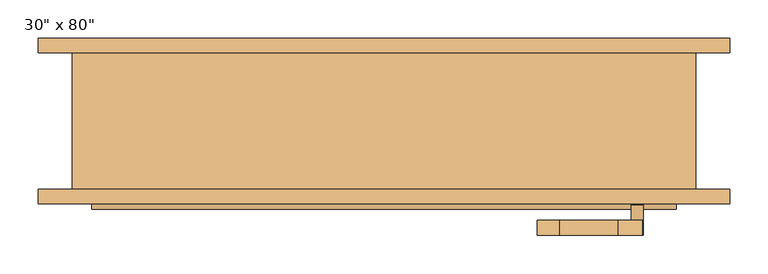
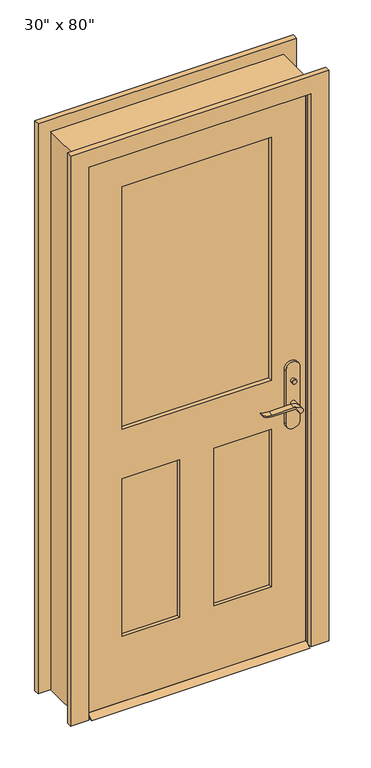
"""IFC4 building model written with IfcOpenShell, lengths in millimetres: door geometry."""

from ifc_helpers import new_model, si_unit, point, frame, frame_2d, origin, place, context, project, spatial, polyline, circle_curve, trimmed, segment, composite_curve, outline, extrude, faceted_brep, source, transform, mapped, element, save


def door_3dfc5bb7(model_context):
    return source(origin(), model_context, "Body", "SolidModel", [
        extrude(outline(polyline([(-50.8, 12.7), (-25.4, 0.0), (-111.125, 0.0), (-85.725, 12.7), (-50.8, 12.7)])), frame((-381.0, 0.0, 0.0), z_axis=(1.0, 0.0, 0.0), x_axis=(0.0, 1.0, 0.0)), (0.0, 0.0, 1.0), 762.0),
        extrude(outline(polyline([(335.2, -30.8), (335.2, -40.8), (325.2, -40.8), (325.2, -30.8), (335.2, -30.8)])), frame((0.0, 0.0, 981.9), z_axis=(0.0, 0.0, 1.0), x_axis=(1.0, 0.0, 0.0)), (0.0, 0.0, 1.0), 30.0),
        extrude(outline(composite_curve([segment(trimmed(circle_curve(frame_2d((996.9, 330.2)), 8.0), [point((996.9, 322.2))], [point((996.9, 338.2))], False, "CARTESIAN"), True, "CONTINUOUS"), segment(trimmed(circle_curve(frame_2d((996.9, 330.2)), 8.0), [point((996.9, 338.2))], [point((996.9, 322.2))], False, "CARTESIAN"), True, "CONTINUOUS")], self_intersect=False)), frame((0.0, -105.725, 0.0), z_axis=(0.0, 1.0, 0.0), x_axis=(0.0, 0.0, 1.0)), (0.0, 0.0, 1.0), 10.0),
        extrude(outline(composite_curve([segment(trimmed(circle_curve(frame_2d((897.1555521, 306.5324871)), 37.2832219), [point((919.0523287, 336.7081363))], [point((934.4, 304.8325667))], False, "CARTESIAN"), True, "CONTINUOUS"), segment(polyline([(934.4, 304.8325667), (934.4, 228.5564091)]), True, "CONTINUOUS"), segment(trimmed(circle_curve(frame_2d((1017.6850638, 228.6227909)), 83.2850902), [point((934.4, 228.5564091))], [point((939.4, 200.2))], True, "CARTESIAN"), True, "CONTINUOUS"), segment(polyline([(939.4, 200.2), (936.6135558, 200.2)]), True, "CONTINUOUS"), segment(trimmed(circle_curve(frame_2d((986.6709207, 232.1396612)), 59.3791355), [point((936.6135558, 200.2))], [point((927.4, 228.5564091))], False, "CARTESIAN"), True, "CONTINUOUS"), segment(polyline([(927.4, 228.5564091), (927.4, 304.8138099)]), True, "CONTINUOUS"), segment(trimmed(circle_curve(frame_2d((909.2738613, 304.8138099)), 18.1261387), [point((927.4, 304.8138099))], [point((914.4, 322.2))], True, "CARTESIAN"), True, "CONTINUOUS"), segment(trimmed(circle_curve(frame_2d((914.4, 330.2)), 8.0), [point((914.4, 322.2))], [point((919.0523287, 336.7081363))], False, "CARTESIAN"), True, "CONTINUOUS")], self_intersect=False)), frame((0.0, -10.8, 0.0), z_axis=(0.0, 1.0, 0.0), x_axis=(0.0, 0.0, 1.0)), (0.0, 0.0, 1.0), 20.0),
        extrude(outline(composite_curve([segment(trimmed(circle_curve(frame_2d((914.4, 330.2)), 8.0), [point((914.3999903, 322.2))], [point((919.0523287, 336.7081363))], False, "CARTESIAN"), True, "CONTINUOUS"), segment(trimmed(circle_curve(frame_2d((897.1555521, 306.5324871)), 37.2832219), [point((919.0523287, 336.7081363))], [point((934.4, 304.8325667))], False, "CARTESIAN"), True, "CONTINUOUS"), segment(polyline([(934.4, 304.8325667), (934.4, 228.5564091)]), True, "CONTINUOUS"), segment(trimmed(circle_curve(frame_2d((1017.6850638, 228.6227909)), 83.2850902), [point((934.4, 228.5564091))], [point((939.4, 200.2))], True, "CARTESIAN"), True, "CONTINUOUS"), segment(polyline([(939.4, 200.2), (936.6135558, 200.2)]), True, "CONTINUOUS"), segment(trimmed(circle_curve(frame_2d((986.6709207, 232.1396612)), 59.3791355), [point((936.6135558, 200.2))], [point((927.4, 228.5564091))], False, "CARTESIAN"), True, "CONTINUOUS"), segment(polyline([(927.4, 228.5564091), (927.4, 304.8138122)]), True, "CONTINUOUS"), segment(trimmed(circle_curve(frame_2d((909.2738682, 304.8138122)), 18.1261318), [point((927.4, 304.8138122))], [point((914.3999903, 322.2))], True, "CARTESIAN"), True, "CONTINUOUS")], self_intersect=False)), frame((0.0, -145.725, 0.0), z_axis=(0.0, 1.0, 0.0), x_axis=(0.0, 0.0, 1.0)), (0.0, 0.0, 1.0), 20.0),
        extrude(outline(composite_curve([segment(trimmed(circle_curve(frame_2d((914.4, 330.2)), 8.0), [point((914.4, 322.2))], [point((914.4, 338.2))], False, "CARTESIAN"), True, "CONTINUOUS"), segment(trimmed(circle_curve(frame_2d((914.4, 330.2)), 8.0), [point((914.4, 338.2))], [point((914.4, 322.2))], False, "CARTESIAN"), True, "CONTINUOUS")], self_intersect=False)), frame((0.0, -40.8, 0.0), z_axis=(0.0, 1.0, 0.0), x_axis=(0.0, 0.0, 1.0)), (0.0, 0.0, 1.0), 30.0),
        extrude(outline(composite_curve([segment(trimmed(circle_curve(frame_2d((914.4, 330.2)), 8.0), [point((914.4, 322.2))], [point((914.4, 338.2))], False, "CARTESIAN"), True, "CONTINUOUS"), segment(trimmed(circle_curve(frame_2d((914.4, 330.2)), 8.0), [point((914.4, 338.2))], [point((914.4, 322.2))], False, "CARTESIAN"), True, "CONTINUOUS")], self_intersect=False)), frame((0.0, -125.725, 0.0), z_axis=(0.0, 1.0, 0.0), x_axis=(0.0, 0.0, 1.0)), (0.0, 0.0, 1.0), 30.0),
        extrude(outline(composite_curve([segment(polyline([(844.4, 355.2), (1039.4, 355.2)]), True, "CONTINUOUS"), segment(trimmed(circle_curve(frame_2d((1039.4, 330.2)), 25.0), [point((1039.4, 355.2))], [point((1039.4, 305.2))], False, "CARTESIAN"), True, "CONTINUOUS"), segment(polyline([(1039.4, 305.2), (844.4, 305.2)]), True, "CONTINUOUS"), segment(trimmed(circle_curve(frame_2d((844.4, 330.2)), 25.0), [point((844.4, 305.2))], [point((844.4, 355.2))], False, "CARTESIAN"), True, "CONTINUOUS")], self_intersect=False)), frame((0.0, -50.8, 0.0), z_axis=(0.0, 1.0, 0.0), x_axis=(0.0, 0.0, 1.0)), (0.0, 0.0, 1.0), 10.0),
        extrude(outline(composite_curve([segment(polyline([(844.4, 355.2), (1039.4, 355.2)]), True, "CONTINUOUS"), segment(trimmed(circle_curve(frame_2d((1039.4, 330.2)), 25.0), [point((1039.4, 355.2))], [point((1039.4, 305.2))], False, "CARTESIAN"), True, "CONTINUOUS"), segment(polyline([(1039.4, 305.2), (844.4, 305.2)]), True, "CONTINUOUS"), segment(trimmed(circle_curve(frame_2d((844.4, 330.2)), 25.0), [point((844.4, 305.2))], [point((844.4, 355.2))], False, "CARTESIAN"), True, "CONTINUOUS")], self_intersect=False)), frame((0.0, -95.725, 0.0), z_axis=(0.0, 1.0, 0.0), x_axis=(0.0, 0.0, 1.0)), (0.0, 0.0, 1.0), 10.0),
        extrude(outline(polyline([(2032.0, -381.0), (12.7, -381.0), (12.7, 381.0), (2032.0, 381.0), (2032.0, -381.0)]), holes=[polyline([(1016.0, -260.35), (1911.35, -260.35), (1911.35, 260.35), (1016.0, 260.35), (1016.0, -260.35)]), polyline([(835.025, -60.325), (254.0, -60.325), (254.0, -260.35), (835.025, -260.35), (835.025, -60.325)]), polyline([(835.025, 260.35), (254.0, 260.35), (254.0, 60.325), (835.025, 60.325), (835.025, 260.35)])]), frame((0.0, -85.725, 0.0), z_axis=(0.0, 1.0, 0.0), x_axis=(0.0, 0.0, 1.0)), (0.0, 0.0, 1.0), 34.925),
        faceted_brep([(406.4, -85.725, 0.0), (381.0, -85.725, 0.0), (381.0, -50.8, 0.0), (368.3, -50.8, 0.0), (368.3, -15.875, 0.0), (381.0, -15.875, 0.0), (381.0, 92.075, 0.0), (406.4, 92.075, 0.0), (406.4, 92.075, 2057.4), (406.4, -85.725, 2057.4), (381.0, 92.075, 2032.0), (-381.0, 92.075, 2032.0), (-381.0, 92.075, 0.0), (-406.4, 92.075, 0.0), (-406.4, 92.075, 2057.4), (381.0, -15.875, 2032.0), (368.3, -15.875, 2019.3), (-368.3, -15.875, 2019.3), (-368.3, -15.875, 0.0), (-381.0, -15.875, 0.0), (-381.0, -15.875, 2032.0), (368.3, -50.8, 2019.3), (381.0, -50.8, 2032.0), (-381.0, -50.8, 2032.0), (-381.0, -50.8, 0.0), (-368.3, -50.8, 0.0), (-368.3, -50.8, 2019.3), (381.0, -85.725, 2032.0), (-406.4, -85.725, 2057.4), (-406.4, -85.725, 0.0), (-381.0, -85.725, 0.0), (-381.0, -85.725, 2032.0)], [[[0, 1, 2, 3, 4, 5, 6, 7]], [[7, 8, 9, 0]], [[6, 10, 11, 12, 13, 14, 8, 7]], [[5, 15, 10, 6]], [[4, 16, 17, 18, 19, 20, 15, 5]], [[3, 21, 16, 4]], [[2, 22, 23, 24, 25, 26, 21, 3]], [[1, 27, 22, 2]], [[0, 9, 28, 29, 30, 31, 27, 1]], [[8, 14, 28, 9]], [[15, 20, 11, 10]], [[21, 26, 17, 16]], [[27, 31, 23, 22]], [[29, 13, 12, 19, 18, 25, 24, 30]], [[14, 13, 29, 28]], [[20, 19, 12, 11]], [[26, 25, 18, 17]], [[31, 30, 24, 23]]]),
        extrude(outline(polyline([(-60.325, -62.4416667), (-60.325, -74.0833333), (-260.35, -74.0833333), (-260.35, -62.4416667), (-60.325, -62.4416667)])), frame((0.0, 0.0, 254.0), z_axis=(0.0, 0.0, 1.0), x_axis=(1.0, 0.0, 0.0)), (0.0, 0.0, 1.0), 581.025),
        extrude(outline(polyline([(260.35, -62.4416667), (260.35, -74.0833333), (60.325, -74.0833333), (60.325, -62.4416667), (260.35, -62.4416667)])), frame((0.0, 0.0, 254.0), z_axis=(0.0, 0.0, 1.0), x_axis=(1.0, 0.0, 0.0)), (0.0, 0.0, 1.0), 581.025),
        extrude(outline(polyline([(260.35, -64.77), (260.35, -71.755), (-260.35, -71.755), (-260.35, -64.77), (260.35, -64.77)])), frame((0.0, 0.0, 1016.0), z_axis=(0.0, 0.0, 1.0), x_axis=(1.0, 0.0, 0.0)), (0.0, 0.0, 1.0), 895.35),
        extrude(outline(polyline([(0.0, -387.35), (2038.35, -387.35), (2038.35, 387.35), (0.0, 387.35), (0.0, 450.85), (2101.85, 450.85), (2101.85, -450.85), (0.0, -450.85), (0.0, -387.35)])), frame((0.0, 92.075, 0.0), z_axis=(0.0, 1.0, 0.0), x_axis=(0.0, 0.0, 1.0)), (0.0, 0.0, 1.0), 19.05),
        extrude(outline(polyline([(0.0, -387.35), (2038.35, -387.35), (2038.35, 387.35), (0.0, 387.35), (0.0, 450.85), (2101.85, 450.85), (2101.85, -450.85), (0.0, -450.85), (0.0, -387.35)])), frame((0.0, -104.775, 0.0), z_axis=(0.0, 1.0, 0.0), x_axis=(0.0, 0.0, 1.0)), (0.0, 0.0, 1.0), 19.05),
    ])


if __name__ == "__main__":
    model = new_model("IFC4")
    model_context = context("Model", 3, world=origin())
    ifc_project = project(units=[si_unit("LENGTHUNIT", "METRE", prefix="MILLI")], contexts=[model_context])
    site = spatial("IfcSite", under=ifc_project)
    building = spatial("IfcBuilding", under=site)
    placement = place(None, origin())
    door_shape = door_3dfc5bb7(model_context)
    element("IfcDoor", 1, ObjectType="30\" x 80\"", at=placement, inside=building, context=model_context, shape_type="MappedRepresentation", body=[
        mapped(door_shape, transform((0.0, 0.0, 0.0), x_axis=(1.0, 0.0, 0.0), y_axis=(0.0, 1.0, 0.0), z_axis=(0.0, 0.0, 1.0))),
    ])
    save(model, "model.ifc")

# Revit data of these elements
# Type "30\" x 80\""
#   Type Mark = "10"
#   Assembly Code = "B2030100"
#   Analytic Construction = "French door, wood frame with single glass"
#   Top Rail = 0' - 4 3/4"
#   Threshold Offset [instance default] = 0' - 0 1/2"
#   Thickness = 0' - 1 3/8"
#   Thermal Resistance (R) = 1.0696 (h·ft²·°F)/BTU
#   Swing Angle [instance default] = 90.00°
#   Stiles = 0' - 4 3/4"
#   Rough Width = 2' - 8"
#   Rough Height = 6' - 9"
#   Lock Rail = 0' - 7 1/8"
#   Height = 6' - 8"
#   Width = 2' - 6"
#   Heat Transfer Coefficient (U) = 0.9350 BTU/(h·ft²·°F)
#   Door Offset [instance default] = 0' - 0"
#   Bottom Rail = 0' - 9 1/2"
#   Threshold [instance default] = yes
#   Function = 1
#   Exterior Trim [instance default] = yes
#   Trim Material = Cherry
#   Threshold Material = Cherry
#   Panel Material = Cherry
#   Glazing = Glass
#   Frame Material = Cherry
#   Door Handle Material = Aluminum
#   Visual Light Transmittance = 0
#   Solar Heat Gain Coefficient = 0
#   Wall Closure = (empty or 0)
#   Construction Type = (empty or 0)
# Element 1 (IfcDoor, "30\" x 80\"")
#   Materials on its faces: "Cherry", "Aluminum", "Glass"
# Materials
#   "Cherry": class "Wood", colour RGB 226 177 128, transparency 0, Description = "Prunus Serotina", Cost = 0
#   "Glass": class "Glass", colour RGB 0 128 192, transparency 0.75, Description = "Soda Lime Glass", Cost = 0
#   "Aluminum": class "Metal", colour RGB 247 247 247, transparency 0, Description = "Aluminum 6061", Cost = 0
